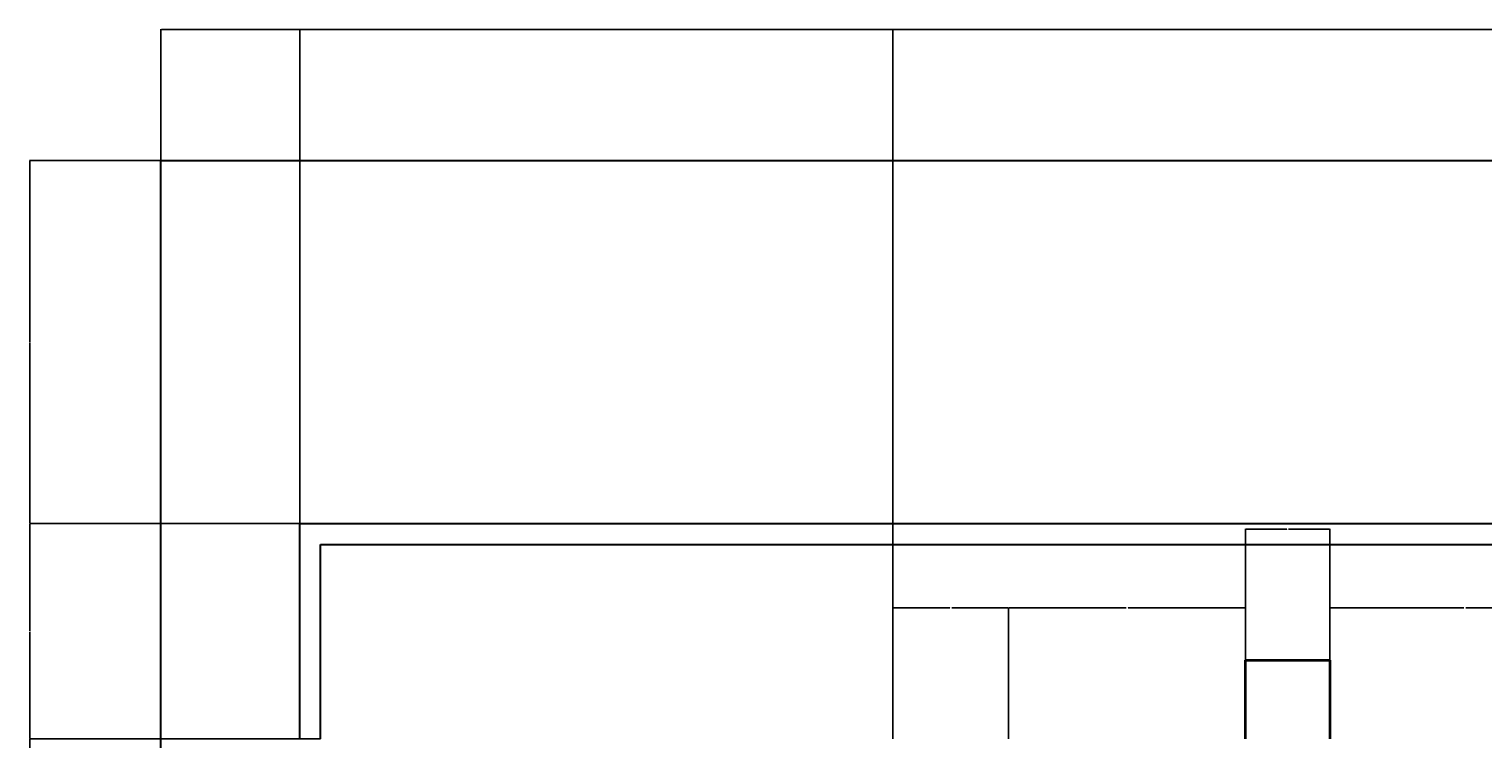
# Model space of a CAD drawing. Units: inches. Extents: x 727 to 1967, y -579 to 606.
# Tile 3 of 5: x 727 to 1355, y 299 to 606. Entities that reach past the tile are written whole.
import ezdxf

# ---------------------------------------------------------------- set-up
doc = ezdxf.new("R2010")
doc.units = ezdxf.units.IN
doc.header["$MEASUREMENT"] = 0
for name, color, linetype, lineweight in [('A-ANNO-DIMS', 2, 'Continuous', 18), ('A-WALL', 7, 'Continuous', 35), ('C-PROP', 7, 'Continuous', 30)]:
    doc.layers.add(name, color=color, linetype=linetype, lineweight=lineweight)
doc.styles.get("Standard").update_dxf_attribs({"font": 'arial.ttf'})
doc.dimstyles.get("Standard").update_dxf_attribs({"dimtxt": 0.18, "dimasz": 0.18, "dimexe": 0.18, "dimexo": 0.0625, "dimgap": 0.09, "dimtad": 0, "dimtih": 1, "dimtoh": 1, "dimdec": 4, "dimzin": 0, "dimdsep": 46, "dimtxsty": 'Standard', "dimcen": 0.09, "dimadec": 0, "dimazin": 0, "dimtfac": 1, "dimtdec": 4, "dimtofl": 0, "dimtmove": 0, "dimatfit": 3, "dimfxl": 1, "dimtolj": 1, "dimtzin": 0, "dimarcsym": 0})

# ---------------------------------------------------------------- blocks, each defined once
blk = doc.blocks.new('*D38')
at = {"layer": 'A-ANNO-DIMS', "color": 0, "lineweight": -2, "transparency": 16777216}
for p, q in [((783.58, 548.95), (783.58, 605.67)), ((783.76, 605.49), (1346.42, 605.49)), ((1910, 605.49), (1347.33, 605.49)), ((1910.18, 548.95), (1910.18, 605.67))]:
    blk.add_line(p, q, dxfattribs=at)
at = {"layer": 'A-ANNO-DIMS', "color": 0, "transparency": 16777216}
for points in [[(783.76, 605.52), (783.76, 605.46), (783.58, 605.49)], [(1910, 605.52), (1910, 605.46), (1910.18, 605.49)]]:
    blk.add_solid(points, dxfattribs=at)
at = {"layer": 'Defpoints', "color": 0, "transparency": 16777216}
for p in [(1910.18, 605.49), (783.58, 548.89), (1910.18, 548.89)]:
    blk.add_point(p, dxfattribs=at)
at = {"layer": 'A-ANNO-DIMS', "color": 0, "transparency": 16777216, "insert": (1346.88, 605.49), "char_height": 0.18, "attachment_point": 5}
blk.add_mtext('\\A1;1126.6', dxfattribs=at)
blk = doc.blocks.new('*D40')
at = {"layer": 'A-ANNO-DIMS', "color": 0, "lineweight": -2, "transparency": 16777216}
for p, q in [((783.58, 392.08), (783.58, 605.67)), ((783.76, 605.49), (813.36, 605.49)), ((843.4, 605.49), (813.8, 605.49)), ((843.58, 392.08), (843.58, 605.67))]:
    blk.add_line(p, q, dxfattribs=at)
at = {"layer": 'A-ANNO-DIMS', "color": 0, "transparency": 16777216}
for points in [[(783.76, 605.52), (783.76, 605.46), (783.58, 605.49)], [(843.4, 605.52), (843.4, 605.46), (843.58, 605.49)]]:
    blk.add_solid(points, dxfattribs=at)
at = {"layer": 'Defpoints', "color": 0, "transparency": 16777216}
for p in [(843.58, 605.49), (783.58, 392.02), (843.58, 392.02)]:
    blk.add_point(p, dxfattribs=at)
at = {"layer": 'A-ANNO-DIMS', "color": 0, "transparency": 16777216, "insert": (813.58, 605.49), "char_height": 0.18, "attachment_point": 5}
blk.add_mtext('\\A1;60', dxfattribs=at)
blk = doc.blocks.new('*D41')
at = {"layer": 'A-ANNO-DIMS', "color": 0, "lineweight": -2, "transparency": 16777216}
for p, q in [((843.58, 392.08), (843.58, 605.67)), ((843.76, 605.49), (971.25, 605.49)), ((1099.67, 605.49), (972.18, 605.49)), ((1099.85, 299.08), (1099.85, 605.67))]:
    blk.add_line(p, q, dxfattribs=at)
at = {"layer": 'A-ANNO-DIMS', "color": 0, "transparency": 16777216}
for points in [[(843.76, 605.52), (843.76, 605.46), (843.58, 605.49)], [(1099.67, 605.52), (1099.67, 605.46), (1099.85, 605.49)]]:
    blk.add_solid(points, dxfattribs=at)
at = {"layer": 'Defpoints', "color": 0, "transparency": 16777216}
for p in [(1099.85, 605.49), (843.58, 392.02), (1099.85, 299.02)]:
    blk.add_point(p, dxfattribs=at)
at = {"layer": 'A-ANNO-DIMS', "color": 0, "transparency": 16777216, "insert": (971.71, 605.49), "char_height": 0.18, "attachment_point": 5}
blk.add_mtext('\\A1;256.26', dxfattribs=at)
blk = doc.blocks.new('*D42')
at = {"layer": 'A-ANNO-DIMS', "color": 0, "lineweight": -2, "transparency": 16777216}
for p, q in [((1099.85, 299.08), (1099.85, 605.67)), ((1100.03, 605.49), (1417.2, 605.49)), ((1735.17, 605.49), (1417.99, 605.49)), ((1735.35, 299.08), (1735.35, 605.67))]:
    blk.add_line(p, q, dxfattribs=at)
at = {"layer": 'A-ANNO-DIMS', "color": 0, "transparency": 16777216}
for points in [[(1100.03, 605.52), (1100.03, 605.46), (1099.85, 605.49)], [(1735.17, 605.52), (1735.17, 605.46), (1735.35, 605.49)]]:
    blk.add_solid(points, dxfattribs=at)
at = {"layer": 'Defpoints', "color": 0, "transparency": 16777216}
for p in [(1735.35, 605.49), (1099.85, 299.02), (1735.35, 299.02)]:
    blk.add_point(p, dxfattribs=at)
at = {"layer": 'A-ANNO-DIMS', "color": 0, "transparency": 16777216, "insert": (1417.6, 605.49), "char_height": 0.18, "attachment_point": 5}
blk.add_mtext('\\A1;635.5', dxfattribs=at)
blk = doc.blocks.new('*D45')
at = {"layer": 'A-ANNO-DIMS', "color": 0, "lineweight": -2, "transparency": 16777216}
for p, q in [((783.52, 548.89), (726.8, 548.89)), ((726.98, 548.71), (726.98, 470.63)), ((726.98, 392.2), (726.98, 470.27)), ((783.52, 392.02), (726.8, 392.02))]:
    blk.add_line(p, q, dxfattribs=at)
at = {"layer": 'A-ANNO-DIMS', "color": 0, "transparency": 16777216}
for points in [[(726.95, 548.71), (727.01, 548.71), (726.98, 548.89)], [(726.95, 392.2), (727.01, 392.2), (726.98, 392.02)]]:
    blk.add_solid(points, dxfattribs=at)
at = {"layer": 'Defpoints', "color": 0, "transparency": 16777216}
for p in [(726.98, 548.89), (783.58, 548.89), (783.58, 392.02)]:
    blk.add_point(p, dxfattribs=at)
at = {"layer": 'A-ANNO-DIMS', "color": 0, "transparency": 16777216, "insert": (726.98, 470.45), "char_height": 0.18, "attachment_point": 5}
blk.add_mtext('\\A1;156.87', dxfattribs=at)
blk = doc.blocks.new('*D46')
at = {"layer": 'A-ANNO-DIMS', "color": 0, "lineweight": -2, "transparency": 16777216}
for p, q in [((843.52, 392.02), (726.8, 392.02)), ((726.98, 391.84), (726.98, 345.7)), ((726.98, 299.2), (726.98, 345.33)), ((852.52, 299.02), (726.8, 299.02))]:
    blk.add_line(p, q, dxfattribs=at)
at = {"layer": 'A-ANNO-DIMS', "color": 0, "transparency": 16777216}
for points in [[(726.95, 391.84), (727.01, 391.84), (726.98, 392.02)], [(726.95, 299.2), (727.01, 299.2), (726.98, 299.02)]]:
    blk.add_solid(points, dxfattribs=at)
at = {"layer": 'Defpoints', "color": 0, "transparency": 16777216}
for p in [(843.58, 392.02), (726.98, 299.02), (852.58, 299.02)]:
    blk.add_point(p, dxfattribs=at)
at = {"layer": 'A-ANNO-DIMS', "color": 0, "transparency": 16777216, "insert": (726.98, 345.52), "char_height": 0.18, "attachment_point": 5}
blk.add_mtext('\\A1;93', dxfattribs=at)
blk = doc.blocks.new('*D47')
at = {"layer": 'A-ANNO-DIMS', "color": 0, "lineweight": -2, "transparency": 16777216}
for p, q in [((852.52, 299.02), (726.8, 299.02)), ((726.98, 298.84), (726.98, 122.7)), ((726.98, -53.8), (726.98, 122.33)), ((852.52, -53.98), (726.8, -53.98))]:
    blk.add_line(p, q, dxfattribs=at)
at = {"layer": 'A-ANNO-DIMS', "color": 0, "transparency": 16777216}
for points in [[(726.95, 298.84), (727.01, 298.84), (726.98, 299.02)], [(726.95, -53.8), (727.01, -53.8), (726.98, -53.98)]]:
    blk.add_solid(points, dxfattribs=at)
at = {"layer": 'Defpoints', "color": 0, "transparency": 16777216}
for p in [(852.58, 299.02), (726.98, -53.98), (852.58, -53.98)]:
    blk.add_point(p, dxfattribs=at)
at = {"layer": 'A-ANNO-DIMS', "color": 0, "transparency": 16777216, "insert": (726.98, 122.52), "char_height": 0.18, "attachment_point": 5}
blk.add_mtext('\\A1;353', dxfattribs=at)
blk = doc.blocks.new('*D54')
at = {"layer": 'A-ANNO-DIMS', "color": 0, "lineweight": -2, "transparency": 16777216}
for p, q in [((1099.85, 299.08), (1099.85, 355.8)), ((1100.03, 355.62), (1124.44, 355.62)), ((1149.64, 355.62), (1125.23, 355.62)), ((1149.82, 299.08), (1149.82, 355.8))]:
    blk.add_line(p, q, dxfattribs=at)
at = {"layer": 'A-ANNO-DIMS', "color": 0, "transparency": 16777216}
for points in [[(1100.03, 355.65), (1100.03, 355.59), (1099.85, 355.62)], [(1149.64, 355.65), (1149.64, 355.59), (1149.82, 355.62)]]:
    blk.add_solid(points, dxfattribs=at)
at = {"layer": 'Defpoints', "color": 0, "transparency": 16777216}
for p in [(1149.82, 355.62), (1099.85, 299.02), (1149.82, 299.02)]:
    blk.add_point(p, dxfattribs=at)
at = {"layer": 'A-ANNO-DIMS', "color": 0, "transparency": 16777216, "insert": (1124.83, 355.62), "char_height": 0.18, "attachment_point": 5}
blk.add_mtext('\\A1;49.97', dxfattribs=at)
blk = doc.blocks.new('*D55')
at = {"layer": 'A-ANNO-DIMS', "color": 0, "lineweight": -2, "transparency": 16777216}
for p, q in [((1149.82, 299.08), (1149.82, 355.8)), ((1150, 355.62), (1200.54, 355.62)), ((1251.99, 355.62), (1201.45, 355.62)), ((1252.17, 299.08), (1252.17, 355.8))]:
    blk.add_line(p, q, dxfattribs=at)
at = {"layer": 'A-ANNO-DIMS', "color": 0, "transparency": 16777216}
for points in [[(1150, 355.65), (1150, 355.59), (1149.82, 355.62)], [(1251.99, 355.65), (1251.99, 355.59), (1252.17, 355.62)]]:
    blk.add_solid(points, dxfattribs=at)
at = {"layer": 'Defpoints', "color": 0, "transparency": 16777216}
for p in [(1252.17, 355.62), (1149.82, 299.02), (1252.17, 299.02)]:
    blk.add_point(p, dxfattribs=at)
at = {"layer": 'A-ANNO-DIMS', "color": 0, "transparency": 16777216, "insert": (1200.99, 355.62), "char_height": 0.18, "attachment_point": 5}
blk.add_mtext('\\A1;102.35', dxfattribs=at)
blk = doc.blocks.new('*D56')
at = {"layer": 'A-ANNO-DIMS', "color": 0, "lineweight": -2, "transparency": 16777216}
for p, q in [((1252.17, 333.09), (1252.17, 389.8)), ((1252.35, 389.62), (1270.01, 389.62)), ((1288.46, 389.62), (1270.8, 389.62)), ((1288.64, 333.09), (1288.64, 389.8))]:
    blk.add_line(p, q, dxfattribs=at)
at = {"layer": 'A-ANNO-DIMS', "color": 0, "transparency": 16777216}
for points in [[(1252.35, 389.65), (1252.35, 389.59), (1252.17, 389.62)], [(1288.46, 389.65), (1288.46, 389.59), (1288.64, 389.62)]]:
    blk.add_solid(points, dxfattribs=at)
at = {"layer": 'Defpoints', "color": 0, "transparency": 16777216}
for p in [(1288.64, 389.62), (1252.17, 333.02), (1288.64, 333.02)]:
    blk.add_point(p, dxfattribs=at)
at = {"layer": 'A-ANNO-DIMS', "color": 0, "transparency": 16777216, "insert": (1270.4, 389.62), "char_height": 0.18, "attachment_point": 5}
blk.add_mtext('\\A1;36.47', dxfattribs=at)
blk = doc.blocks.new('*D57')
at = {"layer": 'A-ANNO-DIMS', "color": 0, "lineweight": -2, "transparency": 16777216}
for p, q in [((1288.64, 299.08), (1288.64, 355.8)), ((1288.82, 355.62), (1346.51, 355.62)), ((1405.1, 355.62), (1347.42, 355.62)), ((1405.28, 299.08), (1405.28, 355.8))]:
    blk.add_line(p, q, dxfattribs=at)
at = {"layer": 'A-ANNO-DIMS', "color": 0, "transparency": 16777216}
for points in [[(1288.82, 355.65), (1288.82, 355.59), (1288.64, 355.62)], [(1405.1, 355.65), (1405.1, 355.59), (1405.28, 355.62)]]:
    blk.add_solid(points, dxfattribs=at)
at = {"layer": 'Defpoints', "color": 0, "transparency": 16777216}
for p in [(1405.28, 355.62), (1288.64, 299.02), (1405.28, 299.02)]:
    blk.add_point(p, dxfattribs=at)
at = {"layer": 'A-ANNO-DIMS', "color": 0, "transparency": 16777216, "insert": (1346.96, 355.62), "char_height": 0.18, "attachment_point": 5}
blk.add_mtext('\\A1;116.65', dxfattribs=at)

msp = doc.modelspace()

# ---------------------------------------------------------------- linework, layer by layer
at = {"layer": 'A-WALL'}
for p, q in [((1252.1653, 299.0151), (1252.1653, 333.0244)), ((1252.1653, 333.0244), (1288.6382, 333.0244)), ((1288.6382, 333.0244), (1288.6382, 299.0151))]:
    msp.add_line(p, q, dxfattribs=at)
at = {"layer": 'C-PROP'}
for p, q in [((783.5815, 392.0151), (783.5815, 548.8891)), ((783.5815, 548.8891), (1910.1781, 548.8891)), ((783.5815, -461.8103), (783.5815, 392.0151)), ((843.5815, 299.0151), (843.5815, 392.0151)), ((843.5815, 392.0151), (1850.1781, 392.0151)), ((852.5815, 359.0151), (852.5815, 383.0151)), ((852.5815, 383.0151), (1841.1781, 383.0151)), ((852.5815, 299.0151), (852.5815, 359.0151))]:
    msp.add_line(p, q, dxfattribs=at)

# ---------------------------------------------------------------- dimensions: what is measured, and where the dimension line sits
at = {"layer": 'A-ANNO-DIMS'}
for base, p1, p2, override, picture, middle in [((1910.1781, 605.4891), (783.5815, 548.8891), (1910.1781, 548.8891), {"dimdec": 1, "dimlfac": 1, "dimrnd": 0, "dimzin": 0, "dimdsep": 46, "dimlunit": 2}, '*D38', (1346.8798, 605.4891)), ((843.5815, 605.4891), (783.5815, 392.0151), (843.5815, 392.0151), {"dimdec": 0, "dimlfac": 1, "dimrnd": 0, "dimzin": 0, "dimdsep": 46, "dimlunit": 2}, '*D40', (813.5815, 605.4891)), ((1099.8463, 605.4891), (843.5815, 392.0151), (1099.8463, 299.0151), {"dimdec": 2, "dimlfac": 1, "dimrnd": 0, "dimzin": 0, "dimdsep": 46, "dimlunit": 2}, '*D41', (971.7139, 605.4891)), ((1735.3463, 605.4891), (1099.8463, 299.0151), (1735.3463, 299.0151), {"dimdec": 1, "dimlfac": 1, "dimrnd": 0, "dimzin": 0, "dimdsep": 46, "dimlunit": 2}, '*D42', (1417.5963, 605.4891)), ((1288.6382, 389.6244), (1252.1653, 333.0244), (1288.6382, 333.0244), {"dimdec": 2, "dimlfac": 1, "dimrnd": 0, "dimzin": 0, "dimdsep": 46, "dimlunit": 2}, '*D56', (1270.4018, 389.6244)), ((1149.8197, 355.6151), (1099.8463, 299.0151), (1149.8197, 299.0151), {"dimdec": 2, "dimlfac": 1, "dimrnd": 0, "dimzin": 0, "dimdsep": 46, "dimlunit": 2}, '*D54', (1124.833, 355.6151)), ((1252.1653, 355.6151), (1149.8197, 299.0151), (1252.1653, 299.0151), {"dimdec": 2, "dimlfac": 1, "dimrnd": 0, "dimzin": 0, "dimdsep": 46, "dimlunit": 2}, '*D55', (1200.9925, 355.6151)), ((1405.2835, 355.6151), (1288.6382, 299.0151), (1405.2835, 299.0151), {"dimdec": 2, "dimlfac": 1, "dimrnd": 0, "dimzin": 0, "dimdsep": 46, "dimlunit": 2}, '*D57', (1346.9609, 355.6151))]:
    dim = msp.add_linear_dim(base=base, p1=p1, p2=p2, dimstyle='Standard', override=override, dxfattribs=at)
    dim.commit()
    dim.dimension.update_dxf_attribs({"geometry": picture, "text_midpoint": middle})
for base, p1, p2, override, picture, middle in [((726.9815, 548.8891), (783.5815, 392.0151), (783.5815, 548.8891), {"dimdec": 2, "dimlfac": 1, "dimrnd": 0, "dimzin": 0, "dimdsep": 46, "dimlunit": 2}, '*D45', (726.9815, 470.4521)), ((726.9815, 299.0151), (843.5815, 392.0151), (852.5815, 299.0151), {"dimdec": 0, "dimlfac": 1, "dimrnd": 0, "dimzin": 0, "dimdsep": 46, "dimlunit": 2}, '*D46', (726.9815, 345.5151)), ((726.9815, -53.9849), (852.5815, 299.0151), (852.5815, -53.9849), {"dimdec": 0, "dimlfac": 1, "dimrnd": 0, "dimzin": 0, "dimdsep": 46, "dimlunit": 2}, '*D47', (726.9815, 122.5151))]:
    dim = msp.add_linear_dim(base=base, p1=p1, p2=p2, angle=90, dimstyle='Standard', override=override, dxfattribs=at)
    dim.commit()
    dim.dimension.update_dxf_attribs({"geometry": picture, "text_midpoint": middle})

doc.saveas('drawing.dxf')
